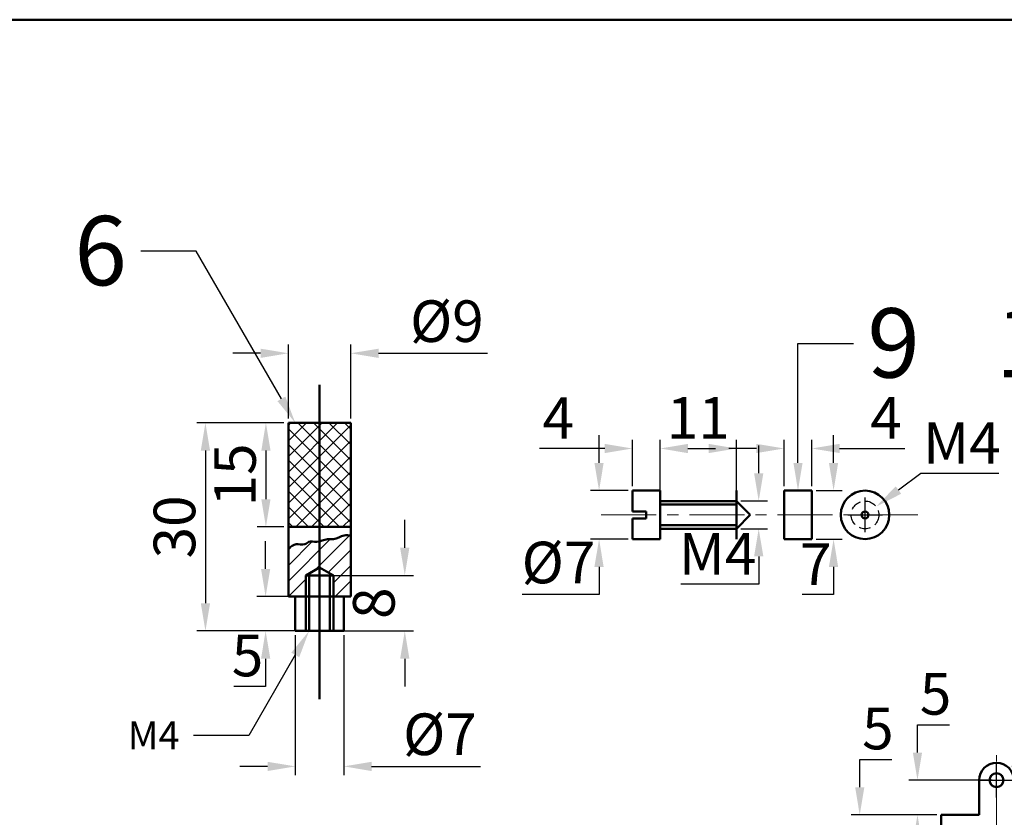
# Model space of a CAD drawing. Units: millimetres. Extents: x 1145 to 1687, y 12 to 400.
# Tile 4 of 6: x 1274 to 1416, y 285 to 400. Entities that reach past the tile are written whole.
import ezdxf
from ezdxf import colors
from ezdxf.entities.mleader import LeaderData, LeaderLine
from ezdxf.math import Vec2, Vec3

# ---------------------------------------------------------------- set-up
doc = ezdxf.new("R2010")
doc.units = ezdxf.units.MM
doc.header["$LTSCALE"] = 0.5
doc.linetypes.add('CENTER', pattern=[50.8, 31.75, -6.35, 6.35, -6.35])
doc.linetypes.add('HIDDEN', pattern=[9.525, 6.35, -3.175])
for name, color, linetype, lineweight in [('M-CNTR', 1, 'CENTER', 18), ('M-DIMS', 2, 'Continuous', 25), ('M-HATC', 8, 'Continuous', 18), ('M-HIDN', 3, 'HIDDEN', 25), ('M-OUTL', 7, 'Continuous', 50), ('M-TEXT', 3, 'Continuous', 25)]:
    doc.layers.add(name, color=color, linetype=linetype, lineweight=lineweight)
doc.styles.get("Standard").update_dxf_attribs({"font": 'arial.ttf'})
doc.dimstyles.new('ISO-25', dxfattribs={"dimtxt": 6, "dimasz": 4, "dimexe": 1.25, "dimexo": 0.625, "dimtad": 1, "dimtoh": 1, "dimdec": 0, "dimtxsty": 'Standard', "dimcen": 2.5, "dimadec": 0, "dimazin": 0, "dimtfac": 1, "dimtdec": 0, "dimtofl": 0, "dimtmove": 0, "dimatfit": 3, "dimfxl": 1, "dimarcsym": 0})

# ---------------------------------------------------------------- blocks, each defined once
blk = doc.blocks.new('*D9')
at = {"layer": 'Defpoints', "color": 0, "ltscale": 0.5, "transparency": 16777216}
for p in [(1321.73, 352.04), (1312.73, 342), (1321.73, 342)]:
    blk.add_point(p, dxfattribs=at)
at = {"layer": 'M-DIMS', "color": 0, "lineweight": -2, "ltscale": 0.5, "transparency": 16777216}
for p, q in [((1312.73, 342.63), (1312.73, 353.29)), ((1321.73, 342.63), (1321.73, 353.29)), ((1308.73, 352.04), (1304.73, 352.04)), ((1325.73, 352.04), (1341.45, 352.04))]:
    blk.add_line(p, q, dxfattribs=at)
at = {"layer": 'M-DIMS', "color": 0, "ltscale": 0.5, "transparency": 16777216}
for points in [[(1308.73, 352.7), (1308.73, 351.37), (1312.73, 352.04)], [(1325.73, 352.7), (1325.73, 351.37), (1321.73, 352.04)]]:
    blk.add_solid(points, dxfattribs=at)
at = {"layer": 'M-DIMS', "color": 0, "ltscale": 0.5, "transparency": 16777216, "insert": (1335.59, 355.89), "char_height": 6, "attachment_point": 5}
blk.add_mtext('%%C9', dxfattribs=at)
blk = doc.blocks.new('*D10')
at = {"layer": 'Defpoints', "color": 0, "ltscale": 0.5, "transparency": 16777216}
for p in [(1313.73, 312), (1320.73, 312), (1320.73, 292.47)]:
    blk.add_point(p, dxfattribs=at)
at = {"layer": 'M-DIMS', "color": 0, "lineweight": -2, "ltscale": 0.5, "transparency": 16777216}
for p, q in [((1313.73, 311.38), (1313.73, 291.22)), ((1320.73, 311.38), (1320.73, 291.22)), ((1309.73, 292.47), (1305.73, 292.47)), ((1324.73, 292.47), (1340.44, 292.47))]:
    blk.add_line(p, q, dxfattribs=at)
at = {"layer": 'M-DIMS', "color": 0, "ltscale": 0.5, "transparency": 16777216}
for points in [[(1309.73, 293.13), (1309.73, 291.8), (1313.73, 292.47)], [(1324.73, 293.13), (1324.73, 291.8), (1320.73, 292.47)]]:
    blk.add_solid(points, dxfattribs=at)
at = {"layer": 'M-DIMS', "color": 0, "ltscale": 0.5, "transparency": 16777216, "insert": (1334.58, 296.32), "char_height": 6, "attachment_point": 5}
blk.add_mtext('%%C7', dxfattribs=at)
blk = doc.blocks.new('*D11')
at = {"layer": 'Defpoints', "color": 0, "ltscale": 0.5, "transparency": 16777216}
for p in [(1312.73, 342), (1300.77, 312), (1313.73, 312)]:
    blk.add_point(p, dxfattribs=at)
at = {"layer": 'M-DIMS', "color": 0, "lineweight": -2, "ltscale": 0.5, "transparency": 16777216}
for p, q in [((1312.1, 342), (1299.52, 342)), ((1300.77, 338), (1300.77, 316)), ((1313.1, 312), (1299.52, 312))]:
    blk.add_line(p, q, dxfattribs=at)
at = {"layer": 'M-DIMS', "color": 0, "ltscale": 0.5, "transparency": 16777216}
for points in [[(1300.1, 338), (1301.44, 338), (1300.77, 342)], [(1300.1, 316), (1301.44, 316), (1300.77, 312)]]:
    blk.add_solid(points, dxfattribs=at)
at = {"layer": 'M-DIMS', "color": 0, "ltscale": 0.5, "transparency": 16777216, "insert": (1297.08, 327), "char_height": 6, "attachment_point": 5, "rotation": 90}
blk.add_mtext('30', dxfattribs=at)
blk = doc.blocks.new('*D12')
at = {"layer": 'Defpoints', "color": 0, "ltscale": 0.5, "transparency": 16777216}
for p in [(1320.73, 316.95), (1309.45, 312), (1320.73, 312)]:
    blk.add_point(p, dxfattribs=at)
at = {"layer": 'M-DIMS', "color": 0, "lineweight": -2, "ltscale": 0.5, "transparency": 16777216}
for p, q in [((1309.45, 320.95), (1309.45, 324.95)), ((1320.1, 316.95), (1308.2, 316.95)), ((1320.1, 312), (1308.2, 312)), ((1309.45, 308), (1309.45, 304)), ((1309.45, 304), (1304.85, 304))]:
    blk.add_line(p, q, dxfattribs=at)
at = {"layer": 'M-DIMS', "color": 0, "ltscale": 0.5, "transparency": 16777216}
for points in [[(1308.79, 320.95), (1310.12, 320.95), (1309.45, 316.95)], [(1308.79, 308), (1310.12, 308), (1309.45, 312)]]:
    blk.add_solid(points, dxfattribs=at)
at = {"layer": 'M-DIMS', "color": 0, "ltscale": 0.5, "transparency": 16777216, "insert": (1306.84, 307.68), "char_height": 6, "attachment_point": 5}
blk.add_mtext('5', dxfattribs=at)
blk = doc.blocks.new('*D13')
at = {"layer": 'Defpoints', "color": 0, "ltscale": 0.5, "transparency": 16777216}
for p in [(1317.23, 320), (1329.52, 320), (1317.23, 312)]:
    blk.add_point(p, dxfattribs=at)
at = {"layer": 'M-DIMS', "color": 0, "lineweight": -2, "ltscale": 0.5, "transparency": 16777216}
for p, q in [((1329.52, 324), (1329.52, 328)), ((1317.85, 320), (1330.77, 320)), ((1317.85, 312), (1330.77, 312)), ((1329.52, 308), (1329.52, 304))]:
    blk.add_line(p, q, dxfattribs=at)
at = {"layer": 'M-DIMS', "color": 0, "ltscale": 0.5, "transparency": 16777216}
for points in [[(1328.85, 324), (1330.18, 324), (1329.52, 320)], [(1328.85, 308), (1330.18, 308), (1329.52, 312)]]:
    blk.add_solid(points, dxfattribs=at)
at = {"layer": 'M-DIMS', "color": 0, "ltscale": 0.5, "transparency": 16777216, "insert": (1325.83, 316), "char_height": 6, "attachment_point": 5, "rotation": 90}
blk.add_mtext('8', dxfattribs=at)
blk = doc.blocks.new('*D14')
at = {"layer": 'Defpoints', "color": 0, "ltscale": 0.5, "transparency": 16777216}
for p in [(1312.73, 342), (1309.49, 327), (1312.73, 327)]:
    blk.add_point(p, dxfattribs=at)
at = {"layer": 'M-DIMS', "color": 0, "lineweight": -2, "ltscale": 0.5, "transparency": 16777216}
for p, q in [((1312.1, 342), (1308.24, 342)), ((1309.49, 338), (1309.49, 331)), ((1312.1, 327), (1308.24, 327))]:
    blk.add_line(p, q, dxfattribs=at)
at = {"layer": 'M-DIMS', "color": 0, "ltscale": 0.5, "transparency": 16777216}
for points in [[(1308.83, 338), (1310.16, 338), (1309.49, 342)], [(1308.83, 331), (1310.16, 331), (1309.49, 327)]]:
    blk.add_solid(points, dxfattribs=at)
at = {"layer": 'M-DIMS', "color": 0, "ltscale": 0.5, "transparency": 16777216, "insert": (1305.81, 334.5), "char_height": 6, "attachment_point": 5, "rotation": 90}
blk.add_mtext('15', dxfattribs=at)
blk = doc.blocks.new('*D15')
at = {"layer": 'Defpoints', "color": 0, "ltscale": 0.5, "transparency": 16777216}
for p in [(1377.35, 338.31), (1366.35, 330.74), (1377.35, 330.74)]:
    blk.add_point(p, dxfattribs=at)
at = {"layer": 'M-DIMS', "color": 0, "lineweight": -2, "ltscale": 0.5, "transparency": 16777216}
for p, q in [((1366.35, 331.36), (1366.35, 339.56)), ((1377.35, 331.36), (1377.35, 339.56)), ((1370.35, 338.31), (1373.35, 338.31))]:
    blk.add_line(p, q, dxfattribs=at)
at = {"layer": 'M-DIMS', "color": 0, "ltscale": 0.5, "transparency": 16777216}
for points in [[(1370.35, 338.97), (1370.35, 337.64), (1366.35, 338.31)], [(1373.35, 338.97), (1373.35, 337.64), (1377.35, 338.31)]]:
    blk.add_solid(points, dxfattribs=at)
at = {"layer": 'M-DIMS', "color": 0, "ltscale": 0.5, "transparency": 16777216, "insert": (1371.85, 341.94), "char_height": 6, "attachment_point": 5}
blk.add_mtext('11', dxfattribs=at)
blk = doc.blocks.new('*D16')
at = {"layer": 'Defpoints', "color": 0, "ltscale": 0.5, "transparency": 16777216}
for p in [(1366.35, 338.31), (1362.35, 332.24), (1366.35, 332.24)]:
    blk.add_point(p, dxfattribs=at)
at = {"layer": 'M-DIMS', "color": 0, "lineweight": -2, "ltscale": 0.5, "transparency": 16777216}
for p, q in [((1362.35, 332.86), (1362.35, 339.56)), ((1366.35, 332.86), (1366.35, 339.56)), ((1358.35, 338.31), (1348.95, 338.31)), ((1370.35, 338.31), (1374.35, 338.31))]:
    blk.add_line(p, q, dxfattribs=at)
at = {"layer": 'M-DIMS', "color": 0, "ltscale": 0.5, "transparency": 16777216}
for points in [[(1358.35, 338.97), (1358.35, 337.64), (1362.35, 338.31)], [(1370.35, 338.97), (1370.35, 337.64), (1366.35, 338.31)]]:
    blk.add_solid(points, dxfattribs=at)
at = {"layer": 'M-DIMS', "color": 0, "ltscale": 0.5, "transparency": 16777216, "insert": (1351.65, 341.93), "char_height": 6, "attachment_point": 5}
blk.add_mtext('4', dxfattribs=at)
blk = doc.blocks.new('*D17')
at = {"layer": 'Defpoints', "color": 0, "ltscale": 0.5, "transparency": 16777216}
for p in [(1377.35, 330.74), (1377.35, 326.74), (1380.56, 326.74)]:
    blk.add_point(p, dxfattribs=at)
at = {"layer": 'M-DIMS', "color": 0, "lineweight": -2, "ltscale": 0.5, "transparency": 16777216}
for p, q in [((1380.56, 334.74), (1380.56, 338.74)), ((1377.97, 330.74), (1381.81, 330.74)), ((1377.97, 326.74), (1381.81, 326.74)), ((1380.56, 322.74), (1380.56, 318.74)), ((1380.56, 318.74), (1369.32, 318.74))]:
    blk.add_line(p, q, dxfattribs=at)
at = {"layer": 'M-DIMS', "color": 0, "ltscale": 0.5, "transparency": 16777216}
for points in [[(1379.9, 334.74), (1381.23, 334.74), (1380.56, 330.74)], [(1379.9, 322.74), (1381.23, 322.74), (1380.56, 326.74)]]:
    blk.add_solid(points, dxfattribs=at)
at = {"layer": 'M-DIMS', "color": 0, "ltscale": 0.5, "transparency": 16777216, "insert": (1374.63, 322.36), "char_height": 6, "attachment_point": 5}
blk.add_mtext('M4', dxfattribs=at)
blk = doc.blocks.new('*D18')
at = {"layer": 'Defpoints', "color": 0, "ltscale": 0.5, "transparency": 16777216}
for p in [(1362.35, 332.24), (1357.54, 325.24), (1362.35, 325.24)]:
    blk.add_point(p, dxfattribs=at)
at = {"layer": 'M-DIMS', "color": 0, "lineweight": -2, "ltscale": 0.5, "transparency": 16777216}
for p, q in [((1357.54, 336.24), (1357.54, 340.24)), ((1361.72, 332.24), (1356.29, 332.24)), ((1361.72, 325.24), (1356.29, 325.24)), ((1357.54, 321.24), (1357.54, 317.24)), ((1357.54, 317.24), (1346.45, 317.24))]:
    blk.add_line(p, q, dxfattribs=at)
at = {"layer": 'M-DIMS', "color": 0, "ltscale": 0.5, "transparency": 16777216}
for points in [[(1356.87, 336.24), (1358.2, 336.24), (1357.54, 332.24)], [(1356.87, 321.24), (1358.2, 321.24), (1357.54, 325.24)]]:
    blk.add_solid(points, dxfattribs=at)
at = {"layer": 'M-DIMS', "color": 0, "ltscale": 0.5, "transparency": 16777216, "insert": (1351.68, 321.09), "char_height": 6, "attachment_point": 5}
blk.add_mtext('%%C7', dxfattribs=at)
blk = doc.blocks.new('*D19')
at = {"layer": 'Defpoints', "color": 0, "ltscale": 0.5, "transparency": 16777216}
for p in [(1388.23, 338.31), (1384.23, 332.24), (1388.23, 332.24)]:
    blk.add_point(p, dxfattribs=at)
at = {"layer": 'M-DIMS', "color": 0, "lineweight": -2, "ltscale": 0.5, "transparency": 16777216}
for p, q in [((1384.23, 332.86), (1384.23, 339.56)), ((1388.23, 332.86), (1388.23, 339.56)), ((1380.23, 338.31), (1376.23, 338.31)), ((1392.23, 338.31), (1401.63, 338.31))]:
    blk.add_line(p, q, dxfattribs=at)
at = {"layer": 'M-DIMS', "color": 0, "ltscale": 0.5, "transparency": 16777216}
for points in [[(1380.23, 338.98), (1380.23, 337.65), (1384.23, 338.31)], [(1392.23, 338.98), (1392.23, 337.65), (1388.23, 338.31)]]:
    blk.add_solid(points, dxfattribs=at)
at = {"layer": 'M-DIMS', "color": 0, "ltscale": 0.5, "transparency": 16777216, "insert": (1398.93, 341.94), "char_height": 6, "attachment_point": 5}
blk.add_mtext('4', dxfattribs=at)
blk = doc.blocks.new('*D20')
at = {"layer": 'Defpoints', "color": 0, "ltscale": 0.5, "transparency": 16777216}
for p in [(1388.23, 332.24), (1388.23, 325.24), (1391.36, 325.24)]:
    blk.add_point(p, dxfattribs=at)
at = {"layer": 'M-DIMS', "color": 0, "lineweight": -2, "ltscale": 0.5, "transparency": 16777216}
for p, q in [((1391.36, 336.24), (1391.36, 340.24)), ((1388.85, 332.24), (1392.61, 332.24)), ((1388.85, 325.24), (1392.61, 325.24)), ((1391.36, 321.24), (1391.36, 317.24)), ((1391.36, 317.24), (1386.85, 317.24))]:
    blk.add_line(p, q, dxfattribs=at)
at = {"layer": 'M-DIMS', "color": 0, "ltscale": 0.5, "transparency": 16777216}
for points in [[(1390.69, 336.24), (1392.02, 336.24), (1391.36, 332.24)], [(1390.69, 321.24), (1392.02, 321.24), (1391.36, 325.24)]]:
    blk.add_solid(points, dxfattribs=at)
at = {"layer": 'M-DIMS', "color": 0, "ltscale": 0.5, "transparency": 16777216, "insert": (1388.79, 320.86), "char_height": 6, "attachment_point": 5}
blk.add_mtext('7', dxfattribs=at)
blk = doc.blocks.new('*D21')
at = {"layer": 'Defpoints', "color": 0, "ltscale": 0.5, "transparency": 16777216}
for p in [(1397.5, 329.93), (1394.29, 327.54)]:
    blk.add_point(p, dxfattribs=at)
at = {"layer": 'M-DIMS', "color": 0, "lineweight": -2, "ltscale": 0.5, "transparency": 16777216}
for p, q in [((1403.93, 334.7), (1400.72, 332.31)), ((1415.17, 334.7), (1403.93, 334.7)), ((1395.9, 326.24), (1395.9, 331.24)), ((1393.4, 328.74), (1398.4, 328.74))]:
    blk.add_line(p, q, dxfattribs=at)
at = {"layer": 'M-DIMS', "color": 0, "ltscale": 0.5, "transparency": 16777216}
blk.add_solid([(1400.32, 332.85), (1401.11, 331.78), (1397.5, 329.93)], dxfattribs=at)
at = {"layer": 'M-DIMS', "color": 0, "ltscale": 0.5, "transparency": 16777216, "insert": (1409.86, 338.32), "char_height": 6, "attachment_point": 5}
blk.add_mtext('M4', dxfattribs=at)
blk = doc.blocks.new('*D43')
at = {"layer": 'Defpoints', "color": 0, "ltscale": 0.5, "transparency": 16777216}
for p in [(1395.13, 285.47), (1406.86, 285.47), (1406.86, 280.47)]:
    blk.add_point(p, dxfattribs=at)
at = {"layer": 'M-DIMS', "color": 0, "lineweight": -2, "ltscale": 0.5, "transparency": 16777216}
for p, q in [((1395.13, 289.47), (1395.13, 293.47)), ((1395.13, 293.47), (1399.74, 293.47)), ((1406.23, 285.47), (1393.88, 285.47)), ((1406.23, 280.47), (1393.88, 280.47)), ((1395.13, 276.47), (1395.13, 272.47))]:
    blk.add_line(p, q, dxfattribs=at)
at = {"layer": 'M-DIMS', "color": 0, "ltscale": 0.5, "transparency": 16777216}
for points in [[(1394.47, 289.47), (1395.8, 289.47), (1395.13, 285.47)], [(1394.47, 276.47), (1395.8, 276.47), (1395.13, 280.47)]]:
    blk.add_solid(points, dxfattribs=at)
at = {"layer": 'M-DIMS', "color": 0, "ltscale": 0.5, "transparency": 16777216, "insert": (1397.75, 297.15), "char_height": 6, "attachment_point": 5}
blk.add_mtext('5', dxfattribs=at)
blk = doc.blocks.new('*D44')
at = {"layer": 'Defpoints', "color": 0, "ltscale": 0.5, "transparency": 16777216}
for p in [(1403.46, 290.47), (1414.86, 290.47), (1406.86, 285.47)]:
    blk.add_point(p, dxfattribs=at)
at = {"layer": 'M-DIMS', "color": 0, "lineweight": -2, "ltscale": 0.5, "transparency": 16777216}
for p, q in [((1403.46, 294.47), (1403.46, 298.47)), ((1403.46, 298.47), (1408.06, 298.47)), ((1414.23, 290.47), (1402.21, 290.47)), ((1406.23, 285.47), (1402.21, 285.47)), ((1403.46, 281.47), (1403.46, 277.47))]:
    blk.add_line(p, q, dxfattribs=at)
at = {"layer": 'M-DIMS', "color": 0, "ltscale": 0.5, "transparency": 16777216}
for points in [[(1402.79, 294.47), (1404.12, 294.47), (1403.46, 290.47)], [(1402.79, 281.47), (1404.12, 281.47), (1403.46, 285.47)]]:
    blk.add_solid(points, dxfattribs=at)
at = {"layer": 'M-DIMS', "color": 0, "ltscale": 0.5, "transparency": 16777216, "insert": (1406.07, 302.15), "char_height": 6, "attachment_point": 5}
blk.add_mtext('5', dxfattribs=at)
blk = doc.blocks.new('*D59')
at = {"layer": 'Defpoints', "color": 0, "ltscale": 0.5, "transparency": 16777216}
for p in [(1416.7, 292.16), (1414.86, 290.47)]:
    blk.add_point(p, dxfattribs=at)
at = {"layer": 'M-DIMS', "color": 0, "lineweight": -2, "ltscale": 0.5, "transparency": 16777216}
for p, q in [((1422.6, 297.56), (1419.65, 294.86)), ((1432.9, 297.56), (1422.6, 297.56)), ((1414.86, 287.97), (1414.86, 292.97)), ((1412.36, 290.47), (1417.36, 290.47))]:
    blk.add_line(p, q, dxfattribs=at)
at = {"layer": 'M-DIMS', "color": 0, "ltscale": 0.5, "transparency": 16777216}
blk.add_solid([(1419.2, 295.35), (1420.1, 294.37), (1416.7, 292.16)], dxfattribs=at)
at = {"layer": 'M-DIMS', "color": 0, "ltscale": 0.5, "transparency": 16777216, "insert": (1428.06, 301.25), "char_height": 6, "attachment_point": 5}
blk.add_mtext('R3', dxfattribs=at)

msp = doc.modelspace()

# ---------------------------------------------------------------- hatches: boundary and pattern name
at = {"layer": 'M-HATC', "ltscale": 0.5}
h = msp.add_hatch(dxfattribs=at)
h.set_pattern_fill('ANSI37', color=256, scale=0.5)
h.set_pattern_definition([(45, (537.9231, 159.5339), (-1.122532, 1.122532), []), (135, (537.9231, 159.5339), (-1.122532, -1.122532), [])])
h.paths.add_polyline_path([(1317.2267, 342.0048), (1312.7267, 342.0048), (1312.7267, 327.0048), (1317.2267, 327.0048)])
h.paths.add_polyline_path([(1321.7267, 342.0048), (1317.2267, 342.0048), (1317.2267, 327.0048), (1321.7267, 327.0048)])
h = msp.add_hatch(dxfattribs=at)
h.set_pattern_fill('ANSI31', color=256, scale=0.5)
h.set_pattern_definition([(45, (537.9231, 159.5339), (-1.122532, 1.122532), [])])
edge = h.paths.add_edge_path()
edge.add_spline(control_points=[(1317.2267, 324.8997), (1317.098, 324.8633), (1316.5848, 324.7611), (1315.7732, 325.0597), (1314.9629, 324.2517), (1313.766, 324.7414), (1313.0784, 324.1521), (1312.7267, 323.8506)], knot_values=[0, 0, 0, 0, 0.39925052, 1.56803338, 2.23250619, 3.47113716, 4.76841242, 4.76841242, 4.76841242, 4.76841242], degree=3, periodic=0)
edge.add_line((1312.7267, 323.8506), (1312.7267, 316.9466))
edge.add_line((1312.7267, 316.9466), (1315.2267, 316.9466))
edge.add_line((1315.2267, 316.9466), (1315.2267, 320.0048))
edge.add_line((1315.2267, 320.0048), (1317.2267, 321.1595))
edge.add_line((1317.2267, 321.1595), (1317.2267, 324.8997))
edge = h.paths.add_edge_path()
edge.add_spline(control_points=[(1321.7267, 325.7633), (1321.4088, 325.7925), (1320.5438, 325.8721), (1319.5168, 325.0999), (1318.2438, 325.3569), (1317.6049, 325.0069), (1317.2267, 324.8997)], knot_values=[4.76841242, 4.76841242, 4.76841242, 4.76841242, 5.70759782, 7.32429458, 8.22969675, 9.40351298, 9.40351298, 9.40351298, 9.40351298], degree=3, periodic=0)
edge.add_line((1317.2267, 324.8997), (1317.2267, 321.1595))
edge.add_line((1317.2267, 321.1595), (1319.2267, 320.0048))
edge.add_line((1319.2267, 320.0048), (1319.2267, 316.9466))
edge.add_line((1319.2267, 316.9466), (1321.7267, 316.9466))
edge.add_line((1321.7267, 316.9466), (1321.7267, 325.7633))

# ---------------------------------------------------------------- linework, layer by layer
at = {"layer": 'M-CNTR', "ltscale": 0.5}
for p, q in [((1357.8588, 328.7357), (1403.5333, 328.7357)), ((1414.8568, 280.4724), (1414.8568, 294.0648))]:
    msp.add_line(p, q, dxfattribs=at)
at = {"layer": 'M-HIDN', "ltscale": 0.5}
msp.add_circle((1395.8993, 328.7357), 2, dxfattribs=at)
at = {"layer": 'M-OUTL', "ltscale": 0.5}
for p, q in [((1317.2267, 302.1669), (1317.2267, 347.5024)), ((1321.7267, 342.0048), (1312.7267, 342.0048)), ((1312.7267, 342.0048), (1312.7267, 316.9466)), ((1313.7267, 342.0048), (1317.2267, 342.0048)), ((1317.2267, 342.0048), (1321.7267, 342.0048)), ((1321.7267, 316.9466), (1321.7267, 342.0048)), ((1362.3455, 332.2357), (1362.3455, 329.2357)), ((1366.3455, 332.2357), (1362.3455, 332.2357)), ((1366.3455, 325.2357), (1366.3455, 332.2357)), ((1377.3455, 325.2357), (1377.3455, 332.2357)), ((1384.2279, 332.2357), (1384.2279, 325.2357)), ((1388.2279, 332.2357), (1384.2279, 332.2357)), ((1388.2279, 325.2357), (1388.2279, 332.2357)), ((1366.3455, 330.7357), (1377.3455, 330.7357)), ((1366.3455, 330.2357), (1377.3455, 330.2357)), ((1379.3438, 328.7357), (1377.3455, 330.7357)), ((1362.3455, 329.2357), (1364.3455, 329.2357)), ((1364.3455, 328.2357), (1362.3455, 328.2357)), ((1362.3455, 328.2357), (1362.3455, 325.2357)), ((1364.3455, 329.2357), (1364.3455, 328.2357)), ((1377.3455, 326.7357), (1379.3438, 328.7357)), ((1321.7267, 327.0048), (1312.7267, 327.0048)), ((1366.3455, 327.2357), (1377.3455, 327.2357)), ((1366.3455, 326.7357), (1377.3455, 326.7357)), ((1362.3455, 325.2357), (1366.3455, 325.2357)), ((1384.2279, 325.2357), (1388.2279, 325.2357)), ((1315.2267, 320.0048), (1317.2267, 321.1595)), ((1319.2267, 320.0048), (1317.2267, 321.1595)), ((1315.2267, 312.0048), (1315.2267, 320.0048)), ((1315.2267, 320.0048), (1319.2267, 320.0048)), ((1315.7267, 312.0048), (1315.7267, 320.0048)), ((1317.2267, 312.0048), (1317.2267, 320.0048)), ((1318.7267, 312.0048), (1318.7267, 320.0048)), ((1319.2267, 312.0048), (1319.2267, 320.0048)), ((1321.7267, 316.9466), (1312.7267, 316.9466)), ((1313.7267, 316.9466), (1320.7267, 316.9466)), ((1313.7267, 312.0048), (1313.7267, 316.9466)), ((1320.7267, 312.0048), (1320.7267, 317.0048)), ((1313.7267, 312.0048), (1320.7267, 312.0048)), ((1412.3568, 290.4724), (1412.3568, 285.4724)), ((1406.8568, 285.4724), (1406.8568, 280.4724)), ((1412.3568, 285.4724), (1406.8568, 285.4724))]:
    msp.add_line(p, q, dxfattribs=at)
msp.add_lwpolyline([(1145.3327, 400.1417), (1687.1285, 400.1417), (1687.1285, 12.2645), (1145.3327, 12.2645)], close=True, dxfattribs=at)
for centre, radius in [((1395.8993, 328.7357), 3.5), ((1395.8993, 328.7357), 0.5), ((1414.8568, 290.4724), 1)]:
    msp.add_circle(centre, radius, dxfattribs=at)
msp.add_arc((1414.8568, 290.4724), 2.5, 0, 180, dxfattribs=at)
msp.add_open_spline([(1312.7267, 323.8506), (1313.0784, 324.1521), (1313.766, 324.7414), (1314.9629, 324.2517), (1315.7732, 325.0597), (1317.0115, 324.6042), (1318.1062, 325.3847), (1319.5168, 325.0999), (1320.5438, 325.8721), (1321.4088, 325.7925), (1321.7267, 325.7633)], degree=3, knots=[0, 0, 0, 0, 1.29727527, 2.53590623, 3.20037904, 4.3691619, 5.94222866, 6.84763082, 8.46432758, 9.40351298, 9.40351298, 9.40351298, 9.40351298], dxfattribs=at)

# ---------------------------------------------------------------- dimensions: what is measured, and where the dimension line sits
at = {"layer": 'M-DIMS', "ltscale": 0.5}
for base, p1, p2, picture, middle in [((1321.7267, 352.0379), (1312.7267, 342.0048), (1321.7267, 342.0048), '*D9', (1335.5883, 355.8942)), ((1320.7267, 292.4651), (1313.7267, 312.0048), (1320.7267, 312.0048), '*D10', (1334.5822, 296.3213))]:
    dim = msp.add_linear_dim(base=base, p1=p1, p2=p2, text='%%C<>', dimstyle='ISO-25', override={"dimclrd": 0, "dimclre": 0, "dimclrt": 0}, dxfattribs=at)
    dim.commit()
    dim.dimension.update_dxf_attribs({"geometry": picture, "text_midpoint": middle})
dim = msp.add_linear_dim(base=(1366.3455, 338.306), p1=(1362.3455, 332.2357), p2=(1366.3455, 332.2357), dimstyle='ISO-25', override={"dimclrd": 0, "dimclre": 0, "dimclrt": 0}, dxfattribs=at)
dim.commit()
dim.dimension.update_dxf_attribs({"geometry": '*D16', "text_midpoint": (1351.6454, 338.306), "dimtype": 160})
for base, p1, p2, picture, middle in [((1377.3455, 338.306), (1366.3455, 330.7357), (1377.3455, 330.7357), '*D15', (1371.8455, 341.9433)), ((1388.2279, 338.3117), (1384.2279, 332.2357), (1388.2279, 332.2357), '*D19', (1398.9279, 341.9367))]:
    dim = msp.add_linear_dim(base=base, p1=p1, p2=p2, dimstyle='ISO-25', override={"dimclrd": 0, "dimclre": 0, "dimclrt": 0}, dxfattribs=at)
    dim.commit()
    dim.dimension.update_dxf_attribs({"geometry": picture, "text_midpoint": middle})
dim = msp.add_diameter_dim_2p(p1=(1394.2939, 327.543), p2=(1397.5048, 329.9284), text='M4', dimstyle='ISO-25', override={"dimclrd": 0, "dimclre": 0, "dimclrt": 0}, dxfattribs=at)
dim.commit()
dim.dimension.update_dxf_attribs({"geometry": '*D21', "text_midpoint": (1409.8598, 338.3243)})
for base, p1, p2, picture, middle in [((1300.7686, 312.0048), (1312.7267, 342.0048), (1313.7267, 312.0048), '*D11', (1300.7686, 327.0048)), ((1391.3574, 325.2357), (1388.2279, 332.2357), (1388.2279, 325.2357), '*D20', (1388.7903, 317.2357))]:
    dim = msp.add_linear_dim(base=base, p1=p1, p2=p2, angle=90, dimstyle='ISO-25', override={"dimclrd": 0, "dimclre": 0, "dimclrt": 0}, dxfattribs=at)
    dim.commit()
    dim.dimension.update_dxf_attribs({"geometry": picture, "text_midpoint": middle, "dimtype": 160})
for base, p1, p2, picture, middle in [((1309.4948, 327.0048), (1312.7267, 342.0048), (1312.7267, 327.0048), '*D14', (1305.8063, 334.5048)), ((1329.5183, 320.0048), (1317.2267, 312.0048), (1317.2267, 320.0048), '*D13', (1325.8298, 316.0048)), ((1309.4532, 312.0048), (1320.7267, 316.9466), (1320.7267, 312.0048), '*D12', (1306.8391, 307.681)), ((1403.4572, 290.4724), (1406.8568, 285.4724), (1414.8568, 290.4724), '*D44', (1406.0712, 302.1485)), ((1395.1331, 285.4724), (1406.8568, 280.4724), (1406.8568, 285.4724), '*D43', (1397.7472, 297.1485))]:
    dim = msp.add_linear_dim(base=base, p1=p1, p2=p2, angle=90, dimstyle='ISO-25', override={"dimclrd": 0, "dimclre": 0, "dimclrt": 0}, dxfattribs=at)
    dim.commit()
    dim.dimension.update_dxf_attribs({"geometry": picture, "text_midpoint": middle})
for base, p1, p2, text, picture, middle in [((1357.5378, 325.2357), (1362.3455, 332.2357), (1362.3455, 325.2357), '%%C<>', '*D18', (1351.6823, 321.092)), ((1380.5635, 326.7357), (1377.3455, 330.7357), (1377.3455, 326.7357), 'M<>', '*D17', (1374.6302, 322.3607))]:
    dim = msp.add_linear_dim(base=base, p1=p1, p2=p2, angle=90, text=text, dimstyle='ISO-25', override={"dimclrd": 0, "dimclre": 0, "dimclrt": 0}, dxfattribs=at)
    dim.commit()
    dim.dimension.update_dxf_attribs({"geometry": picture, "text_midpoint": middle})
dim = msp.add_radius_dim(center=(1414.8568, 290.4724), mpoint=(1416.7007, 292.1606), dimstyle='ISO-25', override={"dimclrd": 0, "dimclre": 0, "dimclrt": 0}, dxfattribs=at)
dim.commit()
dim.dimension.update_dxf_attribs({"geometry": '*D59', "text_midpoint": (1428.0637, 301.2535)})

# ---------------------------------------------------------------- leaders
at = {"layer": 'M-TEXT', "ltscale": 0.5}
ml = msp.add_multileader_mtext('Standard', dxfattribs=at)
ml.set_content('6', color=256)
ml.set_leader_properties()
ml.build(insert=Vec2(0, 0))
ctx = ml.context
ctx.base_point, ctx.char_height, ctx.plane_origin = Vec3(1280.8366, 366.7507), 10, Vec3(1313.7267, 342.0048)
ctx.text_align_type = 2
notes = []
notes.append((ctx, [(0, (1, 1, 0), (1299.4396, 366.7507), (-1, 0), 8, [(0, [(1313.7267, 342.0048)], 0, [])])]))
ctx.mtext.insert, ctx.mtext.alignment, ctx.mtext.flow_direction = Vec3(1289.4396, 371.8359), 3, 5
ml = msp.add_multileader_mtext('Standard', dxfattribs=at)
ml.set_content('9', color=256)
ml.set_leader_properties()
ml.build(insert=Vec2(0, 0))
ctx = ml.context
ctx.base_point, ctx.char_height, ctx.plane_origin = Vec3(1394.2279, 353.4464), 10, Vec3(1386.2279, 332.2357)
notes.append((ctx, [(0, (1, 1, 0), (1386.2279, 353.4464), (1, 0), 8, [(0, [(1386.2279, 332.2357)], 0, [])])]))
ctx.mtext.insert, ctx.mtext.flow_direction = Vec3(1396.2279, 358.5316), 5
ml = msp.add_multileader_mtext('Standard', dxfattribs=at)
ml.set_content('10', color=256)
ml.set_leader_properties()
ml.build(insert=Vec2(0, 0))
ctx = ml.context
ctx.base_point, ctx.char_height, ctx.plane_origin = Vec3(1414.5331, 353.4911), 10, Vec3(1448.7604, 338.1137)
ctx.text_align_type = 2
notes.append((ctx, [(0, (1, 1, 0), (1439.8823, 353.4911), (-1, 0), 8, [(0, [(1448.7604, 338.1137)], 0, [])])]))
ctx.mtext.insert, ctx.mtext.alignment, ctx.mtext.flow_direction = Vec3(1429.8823, 358.5764), 3, 5
ml = msp.add_multileader_mtext('Standard', dxfattribs=at)
ml.set_content('M4', color=256)
ml.set_leader_properties()
ml.build(insert=Vec2(0, 0))
ctx = ml.context
ctx.base_point, ctx.plane_origin = Vec3(1287.9538, 296.9444), Vec3(1315.7267, 312.0048)
ctx.text_align_type = 2
notes.append((ctx, [(0, (1, 1, 0), (1307.0315, 296.9444), (-1, 0), 8, [(0, [(1315.7267, 312.0048)], 0, [])])]))
ctx.mtext.insert, ctx.mtext.alignment, ctx.mtext.flow_direction = Vec3(1297.0315, 298.9444), 3, 5
for ctx, leaders in notes:
    for number, flags, end, landing, length, lines in leaders:
        leader = LeaderData()
        leader.index, (leader.has_last_leader_line, leader.has_dogleg_vector, leader.attachment_direction) = number, flags
        leader.last_leader_point, leader.dogleg_vector, leader.dogleg_length = Vec3(end), Vec3(landing), length
        for number, points, colour, breaks in lines:
            line = LeaderLine()
            line.index, line.vertices, line.color, line.breaks = number, Vec3.list(points), colors.encode_raw_color(colour), breaks
            leader.lines.append(line)
        ctx.leaders.append(leader)

doc.saveas('drawing.dxf')
